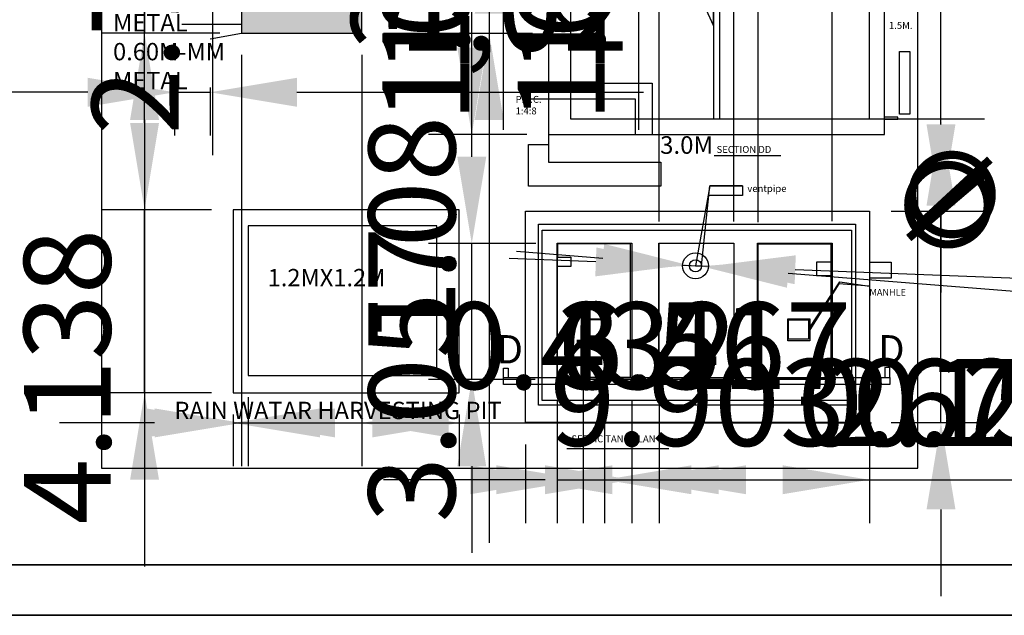
# Model space of a CAD drawing. Units: metres. Extents: x 782 to 1487, y 1262 to 7446.
# Tile 3 of 25: x 821 to 850, y 1262 to 1280. Entities that reach past the tile are written whole.
import ezdxf

# ---------------------------------------------------------------- set-up
doc = ezdxf.new("R2010")
doc.units = ezdxf.units.M
for name, color, linetype, lineweight in [('A-ANNO-DIMS', 2, 'Continuous', 18), ('A-ANNO-TEXT', 3, 'Continuous', 18), ('A-ANNO-TTLB', 7, 'Continuous', 35), ('A-DETL', 7, 'Continuous', 25), ('A-DETL-PATT', 9, 'Continuous', 13)]:
    doc.layers.add(name, color=color, linetype=linetype, lineweight=lineweight)
doc.styles.get("Standard").update_dxf_attribs({"font": 'arial.ttf'})
doc.dimstyles.new('ISO-25', dxfattribs={"dimtxt": 2.5, "dimasz": 2.5, "dimexe": 1.25, "dimexo": 0.625, "dimtad": 1, "dimtxsty": 'Standard', "dimcen": 2.5, "dimadec": 0, "dimazin": 0, "dimtfac": 1, "dimtmove": 0, "dimatfit": 3, "dimfxl": 1, "dimarcsym": 0})

# ---------------------------------------------------------------- blocks, each defined once
blk = doc.blocks.new('*D10')
at = {"layer": 'A-ANNO-DIMS', "color": 0, "lineweight": -2, "transparency": 16777216}
for p, q in [((825.73, 1277.527), (825.73, 1276.166)), ((826.753, 1277.552), (826.753, 1276.166)), ((823.23, 1277.416), (820.73, 1277.416)), ((825.73, 1277.416), (826.753, 1277.416)), ((829.253, 1277.416), (839.235, 1277.416))]:
    blk.add_line(p, q, dxfattribs=at)
at = {"layer": 'A-ANNO-DIMS', "color": 0, "transparency": 16777216}
for points in [[(823.23, 1277.833), (823.23, 1276.999), (825.73, 1277.416)], [(829.253, 1277.833), (829.253, 1276.999), (826.753, 1277.416)]]:
    blk.add_solid(points, dxfattribs=at)
at = {"layer": 'Defpoints', "color": 0, "transparency": 16777216}
for p in [(825.73, 1278.152), (826.753, 1278.177), (826.753, 1277.416)]:
    blk.add_point(p, dxfattribs=at)
at = {"layer": 'A-ANNO-DIMS', "color": 0, "transparency": 16777216, "insert": (835.494, 1279.543), "char_height": 2.5, "attachment_point": 5}
blk.add_mtext('1,02', dxfattribs=at)
blk = doc.blocks.new('*D86')
at = {"layer": 'A-ANNO-DIMS', "color": 0, "lineweight": -2, "transparency": 16777216}
for p, q in [((826.821, 1295.567), (826.821, 1298.067)), ((827.337, 1293.067), (825.571, 1293.067)), ((826.821, 1293.067), (826.821, 1290.305)), ((827.337, 1290.305), (825.571, 1290.305)), ((826.821, 1287.805), (826.821, 1275.602))]:
    blk.add_line(p, q, dxfattribs=at)
at = {"layer": 'A-ANNO-DIMS', "color": 0, "transparency": 16777216}
for points in [[(826.404, 1295.567), (827.238, 1295.567), (826.821, 1293.067)], [(826.404, 1287.805), (827.238, 1287.805), (826.821, 1290.305)]]:
    blk.add_solid(points, dxfattribs=at)
at = {"layer": 'Defpoints', "color": 0, "transparency": 16777216}
for p in [(827.962, 1293.067), (826.821, 1290.305), (827.962, 1290.305)]:
    blk.add_point(p, dxfattribs=at)
at = {"layer": 'A-ANNO-DIMS', "color": 0, "transparency": 16777216, "insert": (824.919, 1280.454), "char_height": 2.5, "attachment_point": 5, "rotation": 90}
blk.add_mtext('2.762', dxfattribs=at)
blk = doc.blocks.new('*D91')
at = {"layer": 'A-ANNO-DIMS', "color": 0, "lineweight": -2, "transparency": 16777216}
for p, q in [((835.19, 1296.199), (835.19, 1298.699)), ((833.037, 1293.699), (836.44, 1293.699)), ((835.19, 1293.699), (835.19, 1293.067)), ((833.037, 1293.067), (836.44, 1293.067)), ((835.19, 1290.567), (835.19, 1278.407))]:
    blk.add_line(p, q, dxfattribs=at)
at = {"layer": 'A-ANNO-DIMS', "color": 0, "transparency": 16777216}
for points in [[(834.774, 1296.199), (835.607, 1296.199), (835.19, 1293.699)], [(834.774, 1290.567), (835.607, 1290.567), (835.19, 1293.067)]]:
    blk.add_solid(points, dxfattribs=at)
at = {"layer": 'Defpoints', "color": 0, "transparency": 16777216}
for p in [(832.412, 1293.699), (832.412, 1293.067), (835.19, 1293.067)]:
    blk.add_point(p, dxfattribs=at)
at = {"layer": 'A-ANNO-DIMS', "color": 0, "transparency": 16777216, "insert": (833.288, 1283.237), "char_height": 2.5, "attachment_point": 5, "rotation": 90}
blk.add_mtext('0.632', dxfattribs=at)
blk = doc.blocks.new('*D92')
at = {"layer": 'A-ANNO-DIMS', "color": 0, "lineweight": -2, "transparency": 16777216}
for p, q in [((835.19, 1295.567), (835.19, 1298.067)), ((831.341, 1293.067), (836.44, 1293.067)), ((835.19, 1293.067), (835.19, 1291.686)), ((831.341, 1291.686), (836.44, 1291.686)), ((835.19, 1289.186), (835.19, 1277.718))]:
    blk.add_line(p, q, dxfattribs=at)
at = {"layer": 'A-ANNO-DIMS', "color": 0, "transparency": 16777216}
for points in [[(834.774, 1295.567), (835.607, 1295.567), (835.19, 1293.067)], [(834.774, 1289.186), (835.607, 1289.186), (835.19, 1291.686)]]:
    blk.add_solid(points, dxfattribs=at)
at = {"layer": 'Defpoints', "color": 0, "transparency": 16777216}
for p in [(830.716, 1293.067), (830.716, 1291.686), (835.19, 1291.686)]:
    blk.add_point(p, dxfattribs=at)
at = {"layer": 'A-ANNO-DIMS', "color": 0, "transparency": 16777216, "insert": (833.288, 1282.202), "char_height": 2.5, "attachment_point": 5, "rotation": 90}
blk.add_mtext('1.381', dxfattribs=at)
blk = doc.blocks.new('*D93')
at = {"layer": 'A-ANNO-DIMS', "color": 0, "lineweight": -2, "transparency": 16777216}
for p, q in [((835.19, 1294.186), (835.19, 1296.686)), ((831.341, 1291.686), (836.44, 1291.686)), ((835.19, 1291.686), (835.19, 1290.305)), ((831.341, 1290.305), (836.44, 1290.305)), ((835.19, 1287.805), (835.19, 1276.337))]:
    blk.add_line(p, q, dxfattribs=at)
at = {"layer": 'A-ANNO-DIMS', "color": 0, "transparency": 16777216}
for points in [[(834.774, 1294.186), (835.607, 1294.186), (835.19, 1291.686)], [(834.774, 1287.805), (835.607, 1287.805), (835.19, 1290.305)]]:
    blk.add_solid(points, dxfattribs=at)
at = {"layer": 'Defpoints', "color": 0, "transparency": 16777216}
for p in [(830.716, 1291.686), (830.716, 1290.305), (835.19, 1290.305)]:
    blk.add_point(p, dxfattribs=at)
at = {"layer": 'A-ANNO-DIMS', "color": 0, "transparency": 16777216, "insert": (833.288, 1280.821), "char_height": 2.5, "attachment_point": 5, "rotation": 90}
blk.add_mtext('1.381', dxfattribs=at)
blk = doc.blocks.new('*D112')
at = {"layer": 'A-ANNO-DIMS', "color": 0, "lineweight": -2, "transparency": 16777216}
for p, q in [((839.091, 1301.615), (839.091, 1304.115)), ((839.466, 1299.115), (837.841, 1299.115)), ((839.091, 1299.115), (839.091, 1293.067)), ((839.466, 1293.067), (837.841, 1293.067)), ((839.091, 1290.567), (839.091, 1278.362))]:
    blk.add_line(p, q, dxfattribs=at)
at = {"layer": 'A-ANNO-DIMS', "color": 0, "transparency": 16777216}
for points in [[(838.675, 1301.615), (839.508, 1301.615), (839.091, 1299.115)], [(838.675, 1290.567), (839.508, 1290.567), (839.091, 1293.067)]]:
    blk.add_solid(points, dxfattribs=at)
at = {"layer": 'Defpoints', "color": 0, "transparency": 16777216}
for p in [(840.091, 1299.115), (839.091, 1293.067), (840.091, 1293.067)]:
    blk.add_point(p, dxfattribs=at)
at = {"layer": 'A-ANNO-DIMS', "color": 0, "transparency": 16777216, "insert": (837.19, 1283.215), "char_height": 2.5, "attachment_point": 5, "rotation": 90}
blk.add_mtext('6.048', dxfattribs=at)
blk = doc.blocks.new('*D113')
at = {"layer": 'A-ANNO-DIMS', "color": 0, "lineweight": -2, "transparency": 16777216}
for p, q in [((839.091, 1295.567), (839.091, 1298.067)), ((839.466, 1293.067), (837.841, 1293.067)), ((839.091, 1293.067), (839.091, 1291.686)), ((839.466, 1291.686), (837.841, 1291.686)), ((839.091, 1289.186), (839.091, 1277.718))]:
    blk.add_line(p, q, dxfattribs=at)
at = {"layer": 'A-ANNO-DIMS', "color": 0, "transparency": 16777216}
for points in [[(838.675, 1295.567), (839.508, 1295.567), (839.091, 1293.067)], [(838.675, 1289.186), (839.508, 1289.186), (839.091, 1291.686)]]:
    blk.add_solid(points, dxfattribs=at)
at = {"layer": 'Defpoints', "color": 0, "transparency": 16777216}
for p in [(840.091, 1293.067), (839.091, 1291.686), (840.091, 1291.686)]:
    blk.add_point(p, dxfattribs=at)
at = {"layer": 'A-ANNO-DIMS', "color": 0, "transparency": 16777216, "insert": (837.189, 1282.202), "char_height": 2.5, "attachment_point": 5, "rotation": 90}
blk.add_mtext('1.381', dxfattribs=at)
blk = doc.blocks.new('*D114')
at = {"layer": 'A-ANNO-DIMS', "color": 0, "lineweight": -2, "transparency": 16777216}
for p, q in [((839.091, 1294.186), (839.091, 1296.686)), ((839.466, 1291.686), (837.841, 1291.686)), ((839.091, 1291.686), (839.091, 1290.305)), ((839.466, 1290.305), (837.841, 1290.305)), ((839.091, 1287.805), (839.091, 1276.337))]:
    blk.add_line(p, q, dxfattribs=at)
at = {"layer": 'A-ANNO-DIMS', "color": 0, "transparency": 16777216}
for points in [[(838.675, 1294.186), (839.508, 1294.186), (839.091, 1291.686)], [(838.675, 1287.805), (839.508, 1287.805), (839.091, 1290.305)]]:
    blk.add_solid(points, dxfattribs=at)
at = {"layer": 'Defpoints', "color": 0, "transparency": 16777216}
for p in [(840.091, 1291.686), (839.091, 1290.305), (840.091, 1290.305)]:
    blk.add_point(p, dxfattribs=at)
at = {"layer": 'A-ANNO-DIMS', "color": 0, "transparency": 16777216, "insert": (837.189, 1280.821), "char_height": 2.5, "attachment_point": 5, "rotation": 90}
blk.add_mtext('1.381', dxfattribs=at)
blk = doc.blocks.new('*D147')
at = {"layer": 'A-ANNO-DIMS', "color": 0, "lineweight": -2, "transparency": 16777216}
for p, q in [((835.84, 1267.272), (835.84, 1265.001)), ((845.743, 1267.272), (845.743, 1265.001)), ((838.34, 1266.251), (843.243, 1266.251))]:
    blk.add_line(p, q, dxfattribs=at)
at = {"layer": 'A-ANNO-DIMS', "color": 0, "transparency": 16777216}
for points in [[(838.34, 1266.668), (838.34, 1265.835), (835.84, 1266.251)], [(843.243, 1266.668), (843.243, 1265.835), (845.743, 1266.251)]]:
    blk.add_solid(points, dxfattribs=at)
at = {"layer": 'Defpoints', "color": 0, "transparency": 16777216}
for p in [(835.84, 1267.897), (845.743, 1267.897), (845.743, 1266.251)]:
    blk.add_point(p, dxfattribs=at)
at = {"layer": 'A-ANNO-DIMS', "color": 0, "transparency": 16777216, "insert": (840.792, 1268.154), "char_height": 2.5, "attachment_point": 5}
blk.add_mtext('9.903', dxfattribs=at)
blk = doc.blocks.new('*D148')
at = {"layer": 'A-ANNO-DIMS', "color": 0, "lineweight": -2, "transparency": 16777216}
for p, q in [((847.802, 1276.491), (847.802, 1288.69)), ((846.368, 1273.991), (849.052, 1273.991)), ((847.802, 1267.897), (847.802, 1273.991)), ((846.368, 1267.897), (849.052, 1267.897)), ((847.802, 1265.397), (847.802, 1262.897))]:
    blk.add_line(p, q, dxfattribs=at)
at = {"layer": 'A-ANNO-DIMS', "color": 0, "transparency": 16777216}
for points in [[(847.386, 1276.491), (848.219, 1276.491), (847.802, 1273.991)], [(847.386, 1265.397), (848.219, 1265.397), (847.802, 1267.897)]]:
    blk.add_solid(points, dxfattribs=at)
at = {"layer": 'Defpoints', "color": 0, "transparency": 16777216}
for p in [(845.743, 1273.991), (847.802, 1273.991), (845.743, 1267.897)]:
    blk.add_point(p, dxfattribs=at)
at = {"layer": 'A-ANNO-DIMS', "color": 0, "transparency": 16777216, "insert": (845.9, 1283.841), "char_height": 2.5, "attachment_point": 5, "rotation": 90}
blk.add_mtext('6.093', dxfattribs=at)
blk = doc.blocks.new('*D149')
at = {"layer": 'A-ANNO-DIMS', "color": 0, "lineweight": -2, "transparency": 16777216}
for p, q in [((836.744, 1268.517), (836.744, 1265.001)), ((838.898, 1268.517), (838.898, 1265.001)), ((834.244, 1266.251), (831.744, 1266.251)), ((836.744, 1266.251), (838.898, 1266.251)), ((841.398, 1266.251), (853.616, 1266.251))]:
    blk.add_line(p, q, dxfattribs=at)
at = {"layer": 'A-ANNO-DIMS', "color": 0, "transparency": 16777216}
for points in [[(834.244, 1266.668), (834.244, 1265.835), (836.744, 1266.251)], [(841.398, 1266.668), (841.398, 1265.835), (838.898, 1266.251)]]:
    blk.add_solid(points, dxfattribs=at)
at = {"layer": 'Defpoints', "color": 0, "transparency": 16777216}
for p in [(836.744, 1269.142), (838.898, 1269.142), (838.898, 1266.251)]:
    blk.add_point(p, dxfattribs=at)
at = {"layer": 'A-ANNO-DIMS', "color": 0, "transparency": 16777216, "insert": (848.757, 1268.153), "char_height": 2.5, "attachment_point": 5}
blk.add_mtext('2.154', dxfattribs=at)
blk = doc.blocks.new('*D150')
at = {"layer": 'A-ANNO-DIMS', "color": 0, "lineweight": -2, "transparency": 16777216}
for p, q in [((838.898, 1268.517), (838.898, 1265.001)), ((839.686, 1268.517), (839.686, 1265.001)), ((836.398, 1266.251), (833.898, 1266.251)), ((838.898, 1266.251), (839.686, 1266.251)), ((842.186, 1266.251), (852.435, 1266.251))]:
    blk.add_line(p, q, dxfattribs=at)
at = {"layer": 'A-ANNO-DIMS', "color": 0, "transparency": 16777216}
for points in [[(836.398, 1266.668), (836.398, 1265.835), (838.898, 1266.251)], [(842.186, 1266.668), (842.186, 1265.835), (839.686, 1266.251)]]:
    blk.add_solid(points, dxfattribs=at)
at = {"layer": 'Defpoints', "color": 0, "transparency": 16777216}
for p in [(838.898, 1269.142), (839.686, 1269.142), (839.686, 1266.251)]:
    blk.add_point(p, dxfattribs=at)
at = {"layer": 'A-ANNO-DIMS', "color": 0, "transparency": 16777216, "insert": (848.561, 1268.153), "char_height": 2.5, "attachment_point": 5}
blk.add_mtext('0.79', dxfattribs=at)
blk = doc.blocks.new('*D151')
at = {"layer": 'A-ANNO-DIMS', "color": 0, "lineweight": -2, "transparency": 16777216}
for p, q in [((839.686, 1273.694), (839.686, 1285.879)), ((841.835, 1273.694), (841.835, 1285.879)), ((837.186, 1284.629), (834.686, 1284.629)), ((839.686, 1284.629), (841.835, 1284.629)), ((844.335, 1284.629), (856.569, 1284.629))]:
    blk.add_line(p, q, dxfattribs=at)
at = {"layer": 'A-ANNO-DIMS', "color": 0, "transparency": 16777216}
for points in [[(837.186, 1285.046), (837.186, 1284.212), (839.686, 1284.629)], [(844.335, 1285.046), (844.335, 1284.212), (841.835, 1284.629)]]:
    blk.add_solid(points, dxfattribs=at)
at = {"layer": 'Defpoints', "color": 0, "transparency": 16777216}
for p in [(841.835, 1284.629), (839.686, 1273.069), (841.835, 1273.069)]:
    blk.add_point(p, dxfattribs=at)
at = {"layer": 'A-ANNO-DIMS', "color": 0, "transparency": 16777216, "insert": (851.702, 1286.531), "char_height": 2.5, "attachment_point": 5}
blk.add_mtext('2.149', dxfattribs=at)
blk = doc.blocks.new('*D152')
at = {"layer": 'A-ANNO-DIMS', "color": 0, "lineweight": -2, "transparency": 16777216}
for p, q in [((841.835, 1273.694), (841.835, 1285.879)), ((842.533, 1273.678), (842.533, 1285.879)), ((839.335, 1284.629), (836.835, 1284.629)), ((841.835, 1284.629), (842.533, 1284.629)), ((845.033, 1284.629), (855.269, 1284.629))]:
    blk.add_line(p, q, dxfattribs=at)
at = {"layer": 'A-ANNO-DIMS', "color": 0, "transparency": 16777216}
for points in [[(839.335, 1285.046), (839.335, 1284.212), (841.835, 1284.629)], [(845.033, 1285.046), (845.033, 1284.212), (842.533, 1284.629)]]:
    blk.add_solid(points, dxfattribs=at)
at = {"layer": 'Defpoints', "color": 0, "transparency": 16777216}
for p in [(842.533, 1284.629), (841.835, 1273.069), (842.533, 1273.053)]:
    blk.add_point(p, dxfattribs=at)
at = {"layer": 'A-ANNO-DIMS', "color": 0, "transparency": 16777216, "insert": (851.401, 1286.531), "char_height": 2.5, "attachment_point": 5}
blk.add_mtext('0.70', dxfattribs=at)
blk = doc.blocks.new('*D153')
at = {"layer": 'A-ANNO-DIMS', "color": 0, "lineweight": -2, "transparency": 16777216}
for p, q in [((842.533, 1273.678), (842.533, 1285.879)), ((844.669, 1273.698), (844.669, 1285.879)), ((840.033, 1284.629), (837.533, 1284.629)), ((842.533, 1284.629), (844.669, 1284.629)), ((847.169, 1284.629), (857.445, 1284.629))]:
    blk.add_line(p, q, dxfattribs=at)
at = {"layer": 'A-ANNO-DIMS', "color": 0, "transparency": 16777216}
for points in [[(840.033, 1285.046), (840.033, 1284.212), (842.533, 1284.629)], [(847.169, 1285.046), (847.169, 1284.212), (844.669, 1284.629)]]:
    blk.add_solid(points, dxfattribs=at)
at = {"layer": 'Defpoints', "color": 0, "transparency": 16777216}
for p in [(844.669, 1284.629), (842.533, 1273.053), (844.669, 1273.073)]:
    blk.add_point(p, dxfattribs=at)
at = {"layer": 'A-ANNO-DIMS', "color": 0, "transparency": 16777216, "insert": (853.557, 1286.509), "char_height": 2.5, "attachment_point": 5}
blk.add_mtext('2.14', dxfattribs=at)
blk = doc.blocks.new('*D154')
at = {"layer": 'A-ANNO-DIMS', "color": 0, "lineweight": -2, "transparency": 16777216}
for p, q in [((834.289, 1275.556), (834.289, 1287.731)), ((836.134, 1273.056), (833.039, 1273.056)), ((834.289, 1269.142), (834.289, 1273.056)), ((836.119, 1269.142), (833.039, 1269.142)), ((834.289, 1266.642), (834.289, 1264.142))]:
    blk.add_line(p, q, dxfattribs=at)
at = {"layer": 'A-ANNO-DIMS', "color": 0, "transparency": 16777216}
for points in [[(833.872, 1275.556), (834.705, 1275.556), (834.289, 1273.056)], [(833.872, 1266.642), (834.705, 1266.642), (834.289, 1269.142)]]:
    blk.add_solid(points, dxfattribs=at)
at = {"layer": 'Defpoints', "color": 0, "transparency": 16777216}
for p in [(834.289, 1273.056), (836.759, 1273.056), (836.744, 1269.142)]:
    blk.add_point(p, dxfattribs=at)
at = {"layer": 'A-ANNO-DIMS', "color": 0, "transparency": 16777216, "insert": (832.386, 1282.893), "char_height": 2.5, "attachment_point": 5, "rotation": 90}
blk.add_mtext('3.914', dxfattribs=at)
blk = doc.blocks.new('*D155')
at = {"layer": 'A-ANNO-DIMS', "color": 0, "lineweight": -2, "transparency": 16777216}
for p, q in [((837.496, 1270.243), (837.496, 1265.001)), ((838.116, 1270.243), (838.116, 1265.001)), ((834.996, 1266.251), (832.496, 1266.251)), ((837.496, 1266.251), (838.116, 1266.251)), ((840.616, 1266.251), (850.834, 1266.251))]:
    blk.add_line(p, q, dxfattribs=at)
at = {"layer": 'A-ANNO-DIMS', "color": 0, "transparency": 16777216}
for points in [[(834.996, 1266.668), (834.996, 1265.835), (837.496, 1266.251)], [(840.616, 1266.668), (840.616, 1265.835), (838.116, 1266.251)]]:
    blk.add_solid(points, dxfattribs=at)
at = {"layer": 'Defpoints', "color": 0, "transparency": 16777216}
for p in [(837.496, 1270.868), (838.116, 1270.868), (838.116, 1266.251)]:
    blk.add_point(p, dxfattribs=at)
at = {"layer": 'A-ANNO-DIMS', "color": 0, "transparency": 16777216, "insert": (846.975, 1268.153), "char_height": 2.5, "attachment_point": 5}
blk.add_mtext('0.62', dxfattribs=at)
blk = doc.blocks.new('*D157')
at = {"layer": 'A-ANNO-DIMS', "color": 0, "lineweight": -2, "transparency": 16777216}
for p, q in [((834.289, 1282.619), (834.289, 1294.819)), ((835.878, 1282.619), (833.039, 1282.619)), ((834.289, 1278.702), (834.289, 1280.119)), ((835.878, 1276.202), (833.039, 1276.202))]:
    blk.add_line(p, q, dxfattribs=at)
at = {"layer": 'A-ANNO-DIMS', "color": 0, "transparency": 16777216}
for points in [[(833.872, 1280.119), (834.705, 1280.119), (834.289, 1282.619)], [(833.872, 1278.702), (834.705, 1278.702), (834.289, 1276.202)]]:
    blk.add_solid(points, dxfattribs=at)
at = {"layer": 'Defpoints', "color": 0, "transparency": 16777216}
for p in [(834.289, 1282.619), (836.503, 1282.619), (836.503, 1276.202)]:
    blk.add_point(p, dxfattribs=at)
at = {"layer": 'A-ANNO-DIMS', "color": 0, "transparency": 16777216, "insert": (832.387, 1289.969), "char_height": 2.5, "attachment_point": 5, "rotation": 90}
blk.add_mtext('6.417', dxfattribs=at)
blk = doc.blocks.new('*D161')
at = {"layer": 'A-ANNO-DIMS', "color": 0, "lineweight": -2, "transparency": 16777216}
for p, q in [((847.802, 1282.319), (847.802, 1294.509)), ((841.88, 1279.819), (849.052, 1279.819)), ((847.802, 1276.651), (847.802, 1279.819)), ((841.88, 1276.651), (849.052, 1276.651)), ((847.802, 1274.151), (847.802, 1271.651))]:
    blk.add_line(p, q, dxfattribs=at)
at = {"layer": 'A-ANNO-DIMS', "color": 0, "transparency": 16777216}
for points in [[(847.386, 1282.319), (848.219, 1282.319), (847.802, 1279.819)], [(847.386, 1274.151), (848.219, 1274.151), (847.802, 1276.651)]]:
    blk.add_solid(points, dxfattribs=at)
at = {"layer": 'Defpoints', "color": 0, "transparency": 16777216}
for p in [(841.255, 1279.819), (847.802, 1279.819), (841.255, 1276.651)]:
    blk.add_point(p, dxfattribs=at)
at = {"layer": 'A-ANNO-DIMS', "color": 0, "transparency": 16777216, "insert": (845.9, 1289.664), "char_height": 2.5, "attachment_point": 5, "rotation": 90}
blk.add_mtext('3.168', dxfattribs=at)
blk = doc.blocks.new('*D162')
at = {"layer": 'A-ANNO-DIMS', "color": 0, "lineweight": -2, "transparency": 16777216}
for p, q in [((827.415, 1268.129), (827.415, 1266.639)), ((829.915, 1267.889), (831.426, 1267.889)), ((833.926, 1268.129), (833.926, 1266.639)), ((833.926, 1267.889), (843.701, 1267.889))]:
    blk.add_line(p, q, dxfattribs=at)
at = {"layer": 'A-ANNO-DIMS', "color": 0, "transparency": 16777216}
for points in [[(829.915, 1268.306), (829.915, 1267.472), (827.415, 1267.889)], [(831.426, 1268.306), (831.426, 1267.472), (833.926, 1267.889)]]:
    blk.add_solid(points, dxfattribs=at)
at = {"layer": 'Defpoints', "color": 0, "transparency": 16777216}
for p in [(827.415, 1268.754), (833.926, 1268.754), (833.926, 1267.889)]:
    blk.add_point(p, dxfattribs=at)
at = {"layer": 'A-ANNO-DIMS', "color": 0, "transparency": 16777216, "insert": (840.063, 1269.79), "char_height": 2.5, "attachment_point": 5}
blk.add_mtext('6.51', dxfattribs=at)
blk = doc.blocks.new('*D163')
at = {"layer": 'A-ANNO-DIMS', "color": 0, "lineweight": -2, "transparency": 16777216}
for p, q in [((824.865, 1276.532), (824.865, 1288.723)), ((826.79, 1274.032), (823.615, 1274.032)), ((824.865, 1268.754), (824.865, 1274.032)), ((826.79, 1268.754), (823.615, 1268.754)), ((824.865, 1266.254), (824.865, 1263.754))]:
    blk.add_line(p, q, dxfattribs=at)
at = {"layer": 'A-ANNO-DIMS', "color": 0, "transparency": 16777216}
for points in [[(824.448, 1276.532), (825.281, 1276.532), (824.865, 1274.032)], [(824.448, 1266.254), (825.281, 1266.254), (824.865, 1268.754)]]:
    blk.add_solid(points, dxfattribs=at)
at = {"layer": 'Defpoints', "color": 0, "transparency": 16777216}
for p in [(824.865, 1274.032), (827.415, 1274.032), (827.415, 1268.754)]:
    blk.add_point(p, dxfattribs=at)
at = {"layer": 'A-ANNO-DIMS', "color": 0, "transparency": 16777216, "insert": (822.963, 1283.878), "char_height": 2.5, "attachment_point": 5, "rotation": 90}
blk.add_mtext('5.278', dxfattribs=at)
blk = doc.blocks.new('*D164')
at = {"layer": 'A-ANNO-DIMS', "color": 0, "lineweight": -2, "transparency": 16777216}
for p, q in [((827.847, 1268.627), (827.847, 1266.639)), ((824.915, 1267.889), (822.415, 1267.889)), ((827.415, 1268.129), (827.415, 1266.639)), ((827.415, 1267.889), (827.847, 1267.889)), ((830.347, 1267.889), (842.508, 1267.889))]:
    blk.add_line(p, q, dxfattribs=at)
at = {"layer": 'A-ANNO-DIMS', "color": 0, "transparency": 16777216}
for points in [[(824.915, 1268.306), (824.915, 1267.472), (827.415, 1267.889)], [(830.347, 1268.306), (830.347, 1267.472), (827.847, 1267.889)]]:
    blk.add_solid(points, dxfattribs=at)
at = {"layer": 'Defpoints', "color": 0, "transparency": 16777216}
for p in [(827.847, 1269.252), (827.415, 1268.754), (827.847, 1267.889)]:
    blk.add_point(p, dxfattribs=at)
at = {"layer": 'A-ANNO-DIMS', "color": 0, "transparency": 16777216, "insert": (837.677, 1269.791), "char_height": 2.5, "attachment_point": 5}
blk.add_mtext('0.432', dxfattribs=at)
blk = doc.blocks.new('*D166')
at = {"layer": 'A-ANNO-DIMS', "color": 0, "lineweight": -2, "transparency": 16777216}
for p, q in [((824.865, 1285.76), (824.865, 1288.26)), ((825.763, 1283.26), (823.615, 1283.26)), ((824.865, 1283.26), (824.865, 1279.121)), ((827.029, 1279.121), (823.615, 1279.121)), ((824.865, 1276.621), (824.865, 1264.329))]:
    blk.add_line(p, q, dxfattribs=at)
at = {"layer": 'A-ANNO-DIMS', "color": 0, "transparency": 16777216}
for points in [[(824.448, 1285.76), (825.281, 1285.76), (824.865, 1283.26)], [(824.448, 1276.621), (825.281, 1276.621), (824.865, 1279.121)]]:
    blk.add_solid(points, dxfattribs=at)
at = {"layer": 'Defpoints', "color": 0, "transparency": 16777216}
for p in [(826.388, 1283.26), (824.865, 1279.121), (827.654, 1279.121)]:
    blk.add_point(p, dxfattribs=at)
at = {"layer": 'A-ANNO-DIMS', "color": 0, "transparency": 16777216, "insert": (822.962, 1269.225), "char_height": 2.5, "attachment_point": 5, "rotation": 90}
blk.add_mtext('4.138', dxfattribs=at)
blk = doc.blocks.new('*D167')
at = {"layer": 'A-ANNO-DIMS', "color": 0, "lineweight": -2, "transparency": 16777216}
for p, q in [((834.791, 1285.76), (834.791, 1288.26)), ((832.636, 1283.26), (836.041, 1283.26)), ((834.791, 1283.26), (834.791, 1282.178)), ((831.746, 1282.178), (836.041, 1282.178)), ((834.791, 1279.678), (834.791, 1269.665))]:
    blk.add_line(p, q, dxfattribs=at)
at = {"layer": 'A-ANNO-DIMS', "color": 0, "transparency": 16777216}
for points in [[(834.374, 1285.76), (835.207, 1285.76), (834.791, 1283.26)], [(834.374, 1279.678), (835.207, 1279.678), (834.791, 1282.178)]]:
    blk.add_solid(points, dxfattribs=at)
at = {"layer": 'Defpoints', "color": 0, "transparency": 16777216}
for p in [(832.011, 1283.26), (831.121, 1282.178), (834.791, 1282.178)]:
    blk.add_point(p, dxfattribs=at)
at = {"layer": 'A-ANNO-DIMS', "color": 0, "transparency": 16777216, "insert": (832.889, 1273.422), "char_height": 2.5, "attachment_point": 5, "rotation": 90}
blk.add_mtext('1.08', dxfattribs=at)
blk = doc.blocks.new('*D168')
at = {"layer": 'A-ANNO-DIMS', "color": 0, "lineweight": -2, "transparency": 16777216}
for p, q in [((834.791, 1284.678), (834.791, 1287.178)), ((831.746, 1282.178), (836.041, 1282.178)), ((834.791, 1282.178), (834.791, 1279.121)), ((831.746, 1279.121), (836.041, 1279.121)), ((834.791, 1276.621), (834.791, 1264.437))]:
    blk.add_line(p, q, dxfattribs=at)
at = {"layer": 'A-ANNO-DIMS', "color": 0, "transparency": 16777216}
for points in [[(834.374, 1284.678), (835.207, 1284.678), (834.791, 1282.178)], [(834.374, 1276.621), (835.207, 1276.621), (834.791, 1279.121)]]:
    blk.add_solid(points, dxfattribs=at)
at = {"layer": 'Defpoints', "color": 0, "transparency": 16777216}
for p in [(831.121, 1282.178), (831.121, 1279.121), (834.791, 1279.121)]:
    blk.add_point(p, dxfattribs=at)
at = {"layer": 'A-ANNO-DIMS', "color": 0, "transparency": 16777216, "insert": (832.888, 1269.279), "char_height": 2.5, "attachment_point": 5, "rotation": 90}
blk.add_mtext('3.057', dxfattribs=at)
blk = doc.blocks.new('*D169')
at = {"layer": 'A-ANNO-DIMS', "color": 0, "lineweight": -2, "transparency": 16777216}
for p, q in [((827.654, 1278.496), (827.654, 1266.639)), ((831.121, 1278.496), (831.121, 1266.639)), ((825.154, 1267.889), (822.654, 1267.889)), ((827.654, 1267.889), (831.121, 1267.889)), ((833.621, 1267.889), (845.805, 1267.889))]:
    blk.add_line(p, q, dxfattribs=at)
at = {"layer": 'A-ANNO-DIMS', "color": 0, "transparency": 16777216}
for points in [[(825.154, 1268.306), (825.154, 1267.472), (827.654, 1267.889)], [(833.621, 1268.306), (833.621, 1267.472), (831.121, 1267.889)]]:
    blk.add_solid(points, dxfattribs=at)
at = {"layer": 'Defpoints', "color": 0, "transparency": 16777216}
for p in [(827.654, 1279.121), (831.121, 1279.121), (831.121, 1267.889)]:
    blk.add_point(p, dxfattribs=at)
at = {"layer": 'A-ANNO-DIMS', "color": 0, "transparency": 16777216, "insert": (840.963, 1269.791), "char_height": 2.5, "attachment_point": 5}
blk.add_mtext('3.467', dxfattribs=at)
blk = doc.blocks.new('*D171')
at = {"layer": 'A-ANNO-DIMS', "color": 0, "lineweight": -2, "transparency": 16777216}
for p, q in [((837.863, 1272.527), (835.364, 1272.625)), ((840.361, 1272.43), (841.106, 1272.401)), ((856.577, 1271.797), (843.604, 1272.303))]:
    blk.add_line(p, q, dxfattribs=at)
at = {"layer": 'A-ANNO-DIMS', "color": 0, "transparency": 16777216}
for points in [[(837.879, 1272.943), (837.846, 1272.111), (840.361, 1272.43)], [(843.621, 1272.719), (843.588, 1271.887), (841.106, 1272.401)]]:
    blk.add_solid(points, dxfattribs=at)
at = {"layer": 'Defpoints', "color": 0, "transparency": 16777216}
for p in [(840.361, 1272.43), (841.106, 1272.401)]:
    blk.add_point(p, dxfattribs=at)
at = {"layer": 'A-ANNO-DIMS', "color": 0, "transparency": 16777216, "insert": (851.417, 1273.971), "char_height": 2.5, "attachment_point": 5, "rotation": 357.7659}
blk.add_mtext('∅0.75', dxfattribs=at)
blk = doc.blocks.new('*D172')
at = {"layer": 'A-ANNO-DIMS', "color": 0, "lineweight": -2, "transparency": 16777216}
for p, q in [((838.066, 1272.631), (835.574, 1272.832)), ((840.558, 1272.429), (840.909, 1272.401)), ((856.341, 1271.153), (843.401, 1272.199))]:
    blk.add_line(p, q, dxfattribs=at)
at = {"layer": 'A-ANNO-DIMS', "color": 0, "transparency": 16777216}
for points in [[(838.1, 1273.046), (838.032, 1272.215), (840.558, 1272.429)], [(843.435, 1272.615), (843.367, 1271.784), (840.909, 1272.401)]]:
    blk.add_solid(points, dxfattribs=at)
at = {"layer": 'Defpoints', "color": 0, "transparency": 16777216}
for p in [(840.558, 1272.429), (840.909, 1272.401)]:
    blk.add_point(p, dxfattribs=at)
at = {"layer": 'A-ANNO-DIMS', "color": 0, "transparency": 16777216, "insert": (851.276, 1273.541), "char_height": 2.5, "attachment_point": 5, "rotation": 355.3781}
blk.add_mtext('∅0.35', dxfattribs=at)

msp = doc.modelspace()

# ---------------------------------------------------------------- hatches: boundary and pattern name
at = {"layer": 'A-DETL-PATT'}
h = msp.add_hatch(color=256, dxfattribs=at)
h.dxf.hatch_style = 1
h.paths.add_polyline_path([(831.1207, 1282.1784), (832.0105, 1282.1784), (832.0105, 1283.2597), (826.3877, 1283.2597), (826.3877, 1282.1784), (827.6538, 1282.1784), (827.6538, 1279.1214), (831.1207, 1279.1214)])
h.paths.add_polyline_path([(823.78, 1277.2166), (828.1675, 1277.2166), (828.1675, 1282.4262), (823.78, 1282.4262)], flags=9)
h = msp.add_hatch(color=256, dxfattribs=at)
h.dxf.hatch_style = 1
h.paths.add_polyline_path([(831.1207, 1282.1784), (832.0105, 1282.1784), (832.0105, 1283.2597), (826.3877, 1283.2597), (826.3877, 1282.1784), (827.6538, 1282.1784), (827.6538, 1279.1214), (831.1207, 1279.1214)])
h.paths.add_polyline_path([(823.78, 1277.2166), (828.1675, 1277.2166), (828.1675, 1282.4262), (823.78, 1282.4262)], flags=9)

# ---------------------------------------------------------------- linework, layer by layer
at = {"layer": 'A-ANNO-TTLB'}
for points in [[(787.4248, 1342.9861), (880.8003, 1342.9861), (880.8003, 1263.8004), (787.4248, 1263.8004)], [(883.6865, 1262.3458), (787.4248, 1262.3458), (787.4248, 1342.9861), (883.6865, 1342.9861)], [(788.8147, 1341.5907), (880.8003, 1341.5907), (880.8003, 1263.8004), (788.8147, 1263.8004)]]:
    msp.add_lwpolyline(points, close=True, dxfattribs=at)
at = {"layer": 'A-DETL'}
for p, q in [((827.6538, 1282.1784), (827.6538, 1279.1214)), ((831.1207, 1279.1214), (831.1207, 1282.1784)), ((840.8283, 1280.2623), (841.2554, 1279.3267)), ((841.2554, 1279.3267), (841.2554, 1279.8192)), ((841.2554, 1279.8192), (841.2554, 1276.6513)), ((841.4362, 1276.6513), (841.4362, 1279.8192)), ((825.9354, 1279.3827), (827.6538, 1279.3827)), ((826.7525, 1278.9538), (827.6538, 1279.1214)), ((827.6538, 1279.1214), (831.1207, 1279.1214)), ((846.6099, 1278.5921), (846.9023, 1278.5921)), ((846.6099, 1276.7853), (846.6099, 1278.5921)), ((846.9023, 1278.5921), (846.9023, 1276.7853)), ((835.8899, 1277.2181), (835.8899, 1277.6778)), ((835.8899, 1277.6778), (839.489, 1277.6778)), ((839.489, 1277.6778), (839.489, 1276.2022)), ((839.0019, 1277.2181), (835.8899, 1277.2181)), ((839.0019, 1276.2022), (839.0019, 1277.2181)), ((846.5581, 1276.6986), (846.1759, 1276.6986)), ((846.5581, 1276.6419), (846.5581, 1276.6986)), ((846.9023, 1276.7853), (846.6099, 1276.7853)), ((841.2554, 1276.6513), (841.4362, 1276.6513)), ((846.1759, 1276.6419), (846.5581, 1276.6419)), ((836.5033, 1276.2022), (839.0019, 1276.2022)), ((836.5033, 1276.2022), (836.5033, 1275.4066)), ((835.925, 1274.707), (835.925, 1275.9086)), ((835.925, 1275.9086), (836.5033, 1275.9086)), ((841.2671, 1275.5909), (843.1912, 1275.5909)), ((836.5033, 1275.4066), (839.7319, 1275.4066)), ((839.7319, 1275.4066), (839.7319, 1274.707)), ((839.7319, 1274.707), (835.925, 1274.707)), ((841.1456, 1274.7242), (840.7335, 1272.4151)), ((840.9097, 1272.4151), (841.1456, 1274.7242)), ((842.0856, 1274.7242), (841.1456, 1274.7242)), ((841.1456, 1274.7242), (842.0856, 1274.7242)), ((842.0856, 1274.7242), (842.0856, 1274.4459)), ((842.0856, 1274.4459), (841.1172, 1274.4459)), ((845.7429, 1273.9906), (845.7429, 1272.5172)), ((836.7592, 1273.0562), (836.7592, 1272.6622)), ((844.633, 1273.0533), (844.633, 1272.521)), ((836.7592, 1272.6622), (837.1438, 1272.6622)), ((837.1438, 1272.6622), (837.1438, 1272.3938)), ((844.633, 1272.521), (844.2192, 1272.521)), ((844.2192, 1272.521), (844.2192, 1272.1365)), ((845.7429, 1272.5172), (846.3666, 1272.5172)), ((846.3666, 1272.5172), (846.3666, 1272.0563)), ((837.1438, 1272.3938), (836.7437, 1272.3938)), ((840.7335, 1272.4151), (840.9097, 1272.4151)), ((844.2192, 1272.1365), (844.633, 1272.1365)), ((844.0281, 1270.6351), (844.8872, 1271.9502)), ((844.8589, 1271.9006), (844.0281, 1270.5697)), ((845.7429, 1271.8298), (844.8589, 1271.9006)), ((844.8872, 1271.9502), (845.7429, 1271.8298)), ((846.3666, 1272.0563), (845.7429, 1272.0563)), ((845.7429, 1272.0563), (845.7429, 1271.8298)), ((844.0281, 1270.8806), (844.0281, 1270.6351)), ((835.2038, 1269.1951), (835.2038, 1269.4699)), ((835.2038, 1269.4699), (835.3338, 1269.4699)), ((835.3338, 1269.4699), (835.3338, 1269.1951)), ((846.3249, 1269.4861), (846.1864, 1269.4861)), ((846.1864, 1269.4861), (846.1864, 1269.1951)), ((846.3249, 1269.1951), (846.3249, 1269.4861)), ((835.1886, 1269.1951), (846.3249, 1269.1951)), ((835.2038, 1268.9934), (835.2038, 1269.1951)), ((846.3249, 1269.1951), (846.3249, 1268.9934)), ((846.3249, 1268.9934), (835.2038, 1268.9934)), ((837.022, 1267.1514), (839.9615, 1267.1514))]:
    msp.add_line(p, q, dxfattribs=at)
for points in [[(823.6278, 1284.0012), (823.6278, 1266.59), (847.1334, 1266.59), (847.1334, 1284.0012)], [(836.5033, 1282.619), (836.5033, 1276.2022), (846.1759, 1276.2022), (846.1759, 1282.619)], [(837.1321, 1282.0186), (837.1321, 1276.6513), (845.7402, 1276.6513), (845.7402, 1282.0186)], [(827.4151, 1274.0318), (827.4151, 1268.754), (833.9257, 1268.754), (833.9257, 1274.0318)], [(835.8402, 1273.9906), (845.7429, 1273.9906), (845.7429, 1267.8971), (835.8402, 1267.8971)], [(827.847, 1273.5678), (827.847, 1269.2516), (833.2787, 1269.2516), (833.2787, 1273.5678)], [(836.2072, 1273.6159), (845.3386, 1273.6159), (845.3386, 1268.3981), (836.2072, 1268.3981)], [(836.3191, 1273.4439), (845.2274, 1273.4439), (845.2274, 1268.5386), (836.3191, 1268.5386)], [(836.7437, 1273.0726), (838.8977, 1273.0726), (838.8977, 1269.1422), (836.7437, 1269.1422)], [(836.7592, 1273.0562), (838.8501, 1273.0562), (838.8501, 1269.1951), (836.7592, 1269.1951)], [(839.681, 1273.0726), (841.835, 1273.0726), (841.835, 1269.1422), (839.681, 1269.1422)], [(839.686, 1273.0692), (841.835, 1273.0692), (841.835, 1269.1422), (839.686, 1269.1422)], [(842.5147, 1273.0726), (844.6687, 1273.0726), (844.6687, 1269.1422), (842.5147, 1269.1422)], [(842.5333, 1273.0533), (844.633, 1273.0533), (844.633, 1269.1793), (842.5333, 1269.1793)], [(837.4767, 1270.8889), (838.1156, 1270.8889), (838.1156, 1270.2505), (837.4767, 1270.2505)], [(837.496, 1270.8681), (838.1156, 1270.8681), (838.1156, 1270.2505), (837.496, 1270.2505)], [(843.3892, 1270.8889), (844.0281, 1270.8889), (844.0281, 1270.2505), (843.3892, 1270.2505)], [(843.4084, 1270.8624), (843.9843, 1270.8624), (843.9843, 1270.2978), (843.4084, 1270.2978)]]:
    msp.add_lwpolyline(points, close=True, dxfattribs=at)
for radius in [0.3731, 0.1762]:
    msp.add_circle((840.7335, 1272.4151), radius, dxfattribs=at)

# ---------------------------------------------------------------- texts
at = {"layer": 'A-ANNO-TEXT', "attachment_point": 1}
for s, width, gutter_width, insert, char_height in [('\\P0.3M. SAND\\P0.60M-20MM METAL\\P0.60M-MM METAL ', 2.795673, 12.5, (823.9569, 1283.0043), 0.5), ('\\P1.5M.', 0.691011, 12.5, (846.3049, 1279.7752), 0.2), ('\\PP.C.C.\\P1:4:8', 1.084166, 12.5, (835.551, 1277.645), 0.2), ('3.0M', 0.080948, 2.5379, (839.7128, 1276.1499), 0.50759), ('\\PSECTION DD', 4.975133, 12.5, (841.3396, 1276.2022), 0.2), ('ventpipe', 2.479081, 12.5, (842.2261, 1274.7421), 0.2), ('1.2MX1.2M', 4.135721, 12.5, (828.4096, 1272.3254), 0.5), ('MANHLE', 1.140238, 12.0231, (845.7429, 1271.7501), 0.19237), ('D ', 0.212907, 4.0731, (834.9993, 1270.4185), 0.81461), ('D ', 0.212907, 4.0731, (845.9904, 1270.4185), 0.81461), ('\\PRAIN WATAR HARVESTING PIT', 10.178586, 12.5, (825.7235, 1269.3325), 0.5), ('SEPTIC TANK PLAN', 9.365252, 12.5, (837.1594, 1267.5302), 0.2)]:
    msp.add_mtext_dynamic_manual_height_columns(s, width=width, gutter_width=gutter_width, heights=[0], dxfattribs=dict(at, insert=insert, char_height=char_height))

# ---------------------------------------------------------------- dimensions: what is measured, and where the dimension line sits
at = {"layer": 'A-ANNO-DIMS'}
for base, p1, p2, override, picture, middle in [((839.0913, 1293.0674), (840.0913, 1299.1153), (840.0913, 1293.0674), {"dimdec": 3, "dimlfac": 1, "dimrnd": 0, "dimzin": 0, "dimdsep": 46, "dimlunit": 2}, '*D112', (837.1899, 1283.2149)), ((835.1905, 1293.0674), (832.4125, 1293.6994), (832.4125, 1293.0674), {"dimdec": 3, "dimlfac": 1, "dimrnd": 0, "dimzin": 0, "dimdsep": 46, "dimlunit": 2}, '*D91', (833.2882, 1283.2371)), ((826.8209, 1290.3053), (827.9625, 1293.0674), (827.9625, 1290.3053), {"dimdec": 3, "dimlfac": 1, "dimrnd": 0, "dimzin": 0, "dimdsep": 46, "dimlunit": 2}, '*D86', (824.9195, 1280.4536)), ((835.1905, 1291.6863), (830.7156, 1293.0674), (830.7156, 1291.6863), {"dimdec": 3, "dimlfac": 1, "dimrnd": 0, "dimzin": 0, "dimdsep": 46, "dimlunit": 2}, '*D92', (833.2882, 1282.2022)), ((839.0913, 1291.6863), (840.0913, 1293.0674), (840.0913, 1291.6863), {"dimdec": 3, "dimlfac": 1, "dimrnd": 0, "dimzin": 0, "dimdsep": 46, "dimlunit": 2}, '*D113', (837.189, 1282.2022)), ((835.1905, 1290.3053), (830.7156, 1291.6863), (830.7156, 1290.3053), {"dimdec": 3, "dimlfac": 1, "dimrnd": 0, "dimzin": 0, "dimdsep": 46, "dimlunit": 2}, '*D93', (833.2882, 1280.8211)), ((839.0913, 1290.3053), (840.0913, 1291.6863), (840.0913, 1290.3053), {"dimdec": 3, "dimlfac": 1, "dimrnd": 0, "dimzin": 0, "dimdsep": 46, "dimlunit": 2}, '*D114', (837.189, 1280.8211)), ((834.2886, 1282.619), (836.5033, 1276.2022), (836.5033, 1282.619), {"dimdec": 3, "dimlfac": 1, "dimrnd": 0, "dimzin": 0, "dimdsep": 46, "dimlunit": 2}, '*D157', (832.3871, 1289.9689)), ((847.8023, 1279.8192), (841.2554, 1276.6513), (841.2554, 1279.8192), {"dimdec": 3, "dimlfac": 1, "dimrnd": 0, "dimzin": 0, "dimdsep": 46, "dimlunit": 2}, '*D161', (845.9, 1289.664)), ((824.8646, 1274.0318), (827.4151, 1268.754), (827.4151, 1274.0318), {"dimdec": 3, "dimlfac": 1, "dimrnd": 0, "dimzin": 0, "dimdsep": 46, "dimlunit": 2}, '*D163', (822.9632, 1283.8775)), ((847.8023, 1273.99059), (845.74287, 1267.89715), (845.74287, 1273.99059), {"dimdec": 3, "dimlfac": 1, "dimrnd": 0, "dimzin": 0, "dimdsep": 46, "dimlunit": 2}, '*D148', (845.90001, 1283.84052)), ((824.8646, 1279.1214), (826.3877, 1283.2597), (827.6538, 1279.1214), {"dimdec": 3, "dimlfac": 1, "dimrnd": 0, "dimzin": 0, "dimdsep": 46, "dimlunit": 2}, '*D166', (822.9623, 1269.2254)), ((834.7907, 1282.1784), (832.0105, 1283.2597), (831.1207, 1282.1784), {"dimdec": 2, "dimlfac": 1, "dimrnd": 0, "dimzin": 0, "dimdsep": 46, "dimlunit": 2}, '*D167', (832.8893, 1273.4216)), ((834.2886, 1273.0562), (836.7437, 1269.1422), (836.7592, 1273.0562), {"dimdec": 3, "dimlfac": 1, "dimrnd": 0, "dimzin": 0, "dimdsep": 46, "dimlunit": 2}, '*D154', (832.3863, 1282.8934)), ((834.7907, 1279.1214), (831.1207, 1282.1784), (831.1207, 1279.1214), {"dimdec": 3, "dimlfac": 1, "dimrnd": 0, "dimzin": 0, "dimdsep": 46, "dimlunit": 2}, '*D168', (832.8885, 1269.2791))]:
    dim = msp.add_linear_dim(base=base, p1=p1, p2=p2, angle=90, dimstyle='ISO-25', override=override, dxfattribs=at)
    dim.commit()
    dim.dimension.update_dxf_attribs({"geometry": picture, "text_midpoint": middle})
for base, p1, p2, override, picture, middle in [((841.835, 1284.6291), (839.686, 1273.0692), (841.835, 1273.0692), {"dimdec": 3, "dimlfac": 1, "dimrnd": 0, "dimzin": 0, "dimdsep": 46, "dimlunit": 2}, '*D151', (851.702, 1286.5306)), ((842.5333, 1284.6291), (841.835, 1273.0692), (842.5333, 1273.0533), {"dimdec": 2, "dimlfac": 1, "dimrnd": 0, "dimzin": 0, "dimdsep": 46, "dimlunit": 2}, '*D152', (851.4009, 1286.5306)), ((844.6687, 1284.6291), (842.5333, 1273.0533), (844.6687, 1273.0726), {"dimdec": 2, "dimlfac": 1, "dimrnd": 0, "dimzin": 0, "dimdsep": 46, "dimlunit": 2}, '*D153', (853.5568, 1286.5093)), ((831.1207, 1267.889), (827.6538, 1279.1214), (831.1207, 1279.1214), {"dimdec": 3, "dimlfac": 1, "dimrnd": 0, "dimzin": 0, "dimdsep": 46, "dimlunit": 2}, '*D169', (840.963, 1269.7913)), ((827.847, 1267.889), (827.4151, 1268.754), (827.847, 1269.2516), {"dimdec": 3, "dimlfac": 1, "dimrnd": 0, "dimzin": 0, "dimdsep": 46, "dimlunit": 2}, '*D164', (837.6774, 1269.7913)), ((833.9257, 1267.889), (827.4151, 1268.754), (833.9257, 1268.754), {"dimdec": 2, "dimlfac": 1, "dimrnd": 0, "dimzin": 0, "dimdsep": 46, "dimlunit": 2}, '*D162', (840.0632, 1269.7905)), ((838.1156, 1266.2514), (837.496, 1270.8681), (838.1156, 1270.8681), {"dimdec": 2, "dimlfac": 1, "dimrnd": 0, "dimzin": 0, "dimdsep": 46, "dimlunit": 2}, '*D155', (846.9747, 1268.1528)), ((838.8977, 1266.2514), (836.7437, 1269.1422), (838.8977, 1269.1422), {"dimdec": 3, "dimlfac": 1, "dimrnd": 0, "dimzin": 0, "dimdsep": 46, "dimlunit": 2}, '*D149', (848.757, 1268.1528)), ((839.686, 1266.2514), (838.8977, 1269.1422), (839.686, 1269.1422), {"dimdec": 2, "dimlfac": 1, "dimrnd": 0, "dimzin": 0, "dimdsep": 46, "dimlunit": 2}, '*D150', (848.5605, 1268.1528)), ((845.7429, 1266.2514), (835.8402, 1267.8971), (845.7429, 1267.8971), {"dimdec": 3, "dimlfac": 1, "dimrnd": 0, "dimzin": 0, "dimdsep": 46, "dimlunit": 2}, '*D147', (840.7915, 1268.1537))]:
    dim = msp.add_linear_dim(base=base, p1=p1, p2=p2, dimstyle='ISO-25', override=override, dxfattribs=at)
    dim.commit()
    dim.dimension.update_dxf_attribs({"geometry": picture, "text_midpoint": middle})
dim = msp.add_linear_dim(base=(826.7525, 1277.4159), p1=(825.7296, 1278.1516), p2=(826.7525, 1278.177), dimstyle='ISO-25', override={"dimclrd": 0, "dimclre": 0, "dimclrt": 0}, dxfattribs=at)
dim.commit()
dim.dimension.update_dxf_attribs({"geometry": '*D10', "text_midpoint": (835.494, 1277.4159), "dimtype": 160})
dim = msp.add_diameter_dim_2p(p1=(840.3606, 1272.4296), p2=(841.1063, 1272.4005), dimstyle='ISO-25', override={"dimdec": 2, "dimlfac": 1, "dimrnd": 0, "dimzin": 0, "dimdsep": 46, "dimlunit": 2}, dxfattribs=at)
dim.commit()
dim.dimension.update_dxf_attribs({"geometry": '*D171', "text_midpoint": (851.3398, 1272.0013)})
dim = msp.add_diameter_dim_2p(p1=(840.5578, 1272.4293), p2=(840.9091, 1272.4009), dimstyle='ISO-25', override={"dimdec": 2, "dimlfac": 1, "dimrnd": 0, "dimzin": 0, "dimdsep": 46, "dimlunit": 2}, dxfattribs=at)
dim.commit()
dim.dimension.update_dxf_attribs({"geometry": '*D172', "text_midpoint": (851.1171, 1271.5756), "dimtype": 163})

doc.saveas('drawing.dxf')
